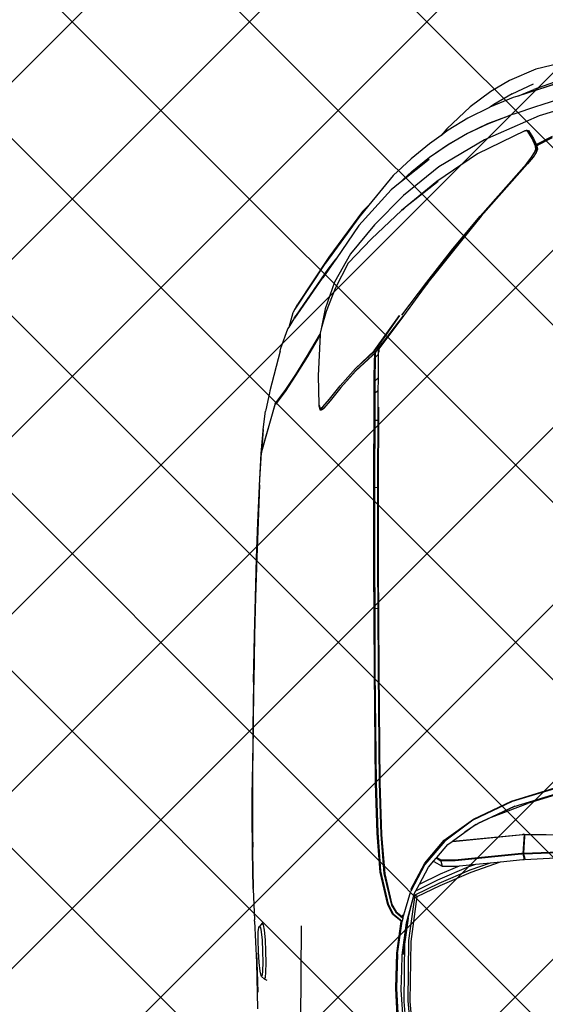
# Model space of a CAD drawing. Units: inches. Extents: x 2167 to 2589, y 1680 to 2489.
# Tile 25 of 38: x 2335 to 2356, y 1796 to 1835. Entities that reach past the tile are written whole.
import ezdxf

# ---------------------------------------------------------------- set-up
doc = ezdxf.new("R2010")
doc.units = ezdxf.units.IN
doc.header["$MEASUREMENT"] = 0
doc.layers.get('0').update_dxf_attribs({"color": 250})
doc.layers.add('C-PRKG-VEHS', color=8, linetype='Continuous', lineweight=13)
doc.layers.add('L-PVMT-PATT', color=252, linetype='Continuous', lineweight=13)
doc.layers.add('Edges', color=250, linetype='Continuous')

# ---------------------------------------------------------------- blocks, each defined once
blk = doc.blocks.new('Nissan Qashqai pl')
at = {"layer": 'Edges'}
for p, q in [((8.4086, 11.6764), (8.4045, 11.4011)), ((8.4305, 11.3996), (8.419, 11.6758)), ((8.4204, 11.6758), (8.4319, 11.3996)), ((8.4394, 11.4014), (8.4238, 11.6766)), ((7.3676, 11.5172), (7.3963, 11.4215)), ((8.3392, 11.4758), (8.3608, 11.4048)), ((7.3193, 11.4645), (7.3309, 11.4166)), ((8.3573, 11.3824), (8.3296, 11.4739)), ((8.3311, 11.4733), (8.3582, 11.3836)), ((8.3648, 11.3863), (8.3377, 11.4753)), ((7.344, 11.4572), (7.3596, 11.4139)), ((7.3467, 11.4596), (7.3686, 11.3913)), ((7.3489, 11.4517), (7.3686, 11.3913)), ((7.375, 11.4442), (7.3799, 11.4278)), ((7.4255, 11.4398), (7.4367, 11.4174)), ((7.4379, 11.4179), (7.4267, 11.4401)), ((8.4041, 11.4013), (8.4048, 11.4423)), ((7.3799, 11.4278), (7.3845, 11.4136)), ((7.3963, 11.4215), (7.4302, 11.3449)), ((7.3309, 11.4166), (7.347, 11.3798)), ((7.3655, 11.3837), (7.3514, 11.4133)), ((7.3686, 11.3913), (7.3596, 11.4139)), ((7.3845, 11.4136), (7.3925, 11.3899)), ((7.4282, 11.4113), (7.4169, 11.4044)), ((7.417, 11.4065), (7.4283, 11.4135)), ((7.4296, 11.4129), (7.4183, 11.406)), ((7.4387, 11.4162), (7.4282, 11.4113)), ((7.4283, 11.4135), (7.4359, 11.417)), ((7.4296, 11.4129), (7.4383, 11.417)), ((7.4359, 11.417), (7.4367, 11.4174)), ((7.4383, 11.417), (7.4367, 11.4174)), ((7.4375, 11.42), (7.4384, 11.4182)), ((7.4379, 11.4179), (7.4384, 11.4182)), ((7.4389, 11.4173), (7.4379, 11.4179)), ((7.4383, 11.417), (7.4379, 11.4179)), ((7.4389, 11.4173), (7.4383, 11.417)), ((7.4384, 11.4182), (7.4387, 11.4183)), ((7.4387, 11.4183), (7.443, 11.4188)), ((7.4431, 11.4166), (7.4387, 11.4162)), ((7.4389, 11.4173), (7.44, 11.4178)), ((7.4442, 11.4183), (7.44, 11.4178)), ((7.443, 11.4188), (7.4477, 11.4172)), ((7.4479, 11.4149), (7.4431, 11.4166)), ((7.4477, 11.4172), (7.4442, 11.4183)), ((7.4477, 11.4172), (7.4541, 11.4128)), ((7.4541, 11.4108), (7.4479, 11.4149)), ((7.4541, 11.4128), (7.4638, 11.4051)), ((7.4635, 11.4034), (7.4541, 11.4108)), ((7.4167, 11.4049), (7.417, 11.4065)), ((7.4172, 11.4047), (7.4167, 11.4049)), ((7.4169, 11.4036), (7.4167, 11.4049)), ((7.4172, 11.4047), (7.4169, 11.4044)), ((7.4169, 11.4044), (7.4169, 11.4036)), ((7.4172, 11.4018), (7.4169, 11.4036)), ((7.4169, 11.4036), (7.4169, 11.403)), ((7.4169, 11.403), (7.4172, 11.4011)), ((7.4183, 11.406), (7.4172, 11.4047)), ((7.4174, 11.4013), (7.4172, 11.4018)), ((7.4172, 11.4011), (7.4498, 11.3349)), ((7.4174, 11.4013), (7.4175, 11.4012)), ((7.5369, 11.3385), (7.4635, 11.4034)), ((7.4638, 11.4051), (7.5371, 11.34)), ((8.3799, 11.3545), (8.3608, 11.4048)), ((8.407, 11.401), (8.4037, 11.4002)), ((8.4037, 11.4002), (8.4314, 11.3985)), ((8.4037, 11.3992), (8.4037, 11.4002)), ((8.4037, 11.3992), (8.4046, 11.3981)), ((8.4042, 11.3983), (8.4037, 11.3992)), ((8.4041, 11.4013), (8.4045, 11.4011)), ((8.4134, 11.3049), (8.4042, 11.3983)), ((8.4045, 11.4011), (8.407, 11.401)), ((8.4046, 11.3981), (8.4138, 11.3048)), ((8.407, 11.401), (8.4305, 11.3996)), ((8.4305, 11.3996), (8.4319, 11.3996)), ((8.4306, 11.3966), (8.4314, 11.3975)), ((8.4398, 11.3032), (8.4306, 11.3966)), ((8.4314, 11.3985), (8.4394, 11.4004)), ((8.4314, 11.3985), (8.4314, 11.3975)), ((8.4314, 11.3975), (8.4319, 11.3967)), ((8.4319, 11.3996), (8.436, 11.4006)), ((8.4319, 11.3967), (8.4412, 11.3033)), ((8.436, 11.4006), (8.4394, 11.4014)), ((8.4394, 11.4004), (8.436, 11.4006)), ((8.4394, 11.3984), (8.4394, 11.4004)), ((8.4425, 11.3672), (8.4394, 11.3984)), ((7.347, 11.3798), (7.3624, 11.3535)), ((7.3655, 11.3837), (7.3805, 11.3576)), ((7.3686, 11.3913), (7.3707, 11.3849)), ((7.3707, 11.3849), (7.3843, 11.3522)), ((7.3925, 11.3899), (7.3938, 11.3859)), ((7.3938, 11.3859), (7.3951, 11.3822)), ((7.3951, 11.3822), (7.3965, 11.3787)), ((8.3826, 11.3291), (8.3573, 11.3824)), ((8.3582, 11.3836), (8.3844, 11.3284)), ((8.3646, 11.387), (8.3799, 11.3545)), ((8.3888, 11.3355), (8.3648, 11.3863)), ((7.3962, 11.3781), (7.3965, 11.3787)), ((7.4071, 11.3493), (7.3962, 11.3781)), ((7.3965, 11.3787), (7.3969, 11.3777)), ((7.3969, 11.3777), (7.4078, 11.349)), ((8.4571, 11.3258), (8.4425, 11.3672)), ((8.4439, 11.3531), (8.4425, 11.3672)), ((7.3624, 11.3535), (7.3837, 11.3245)), ((7.3805, 11.3576), (7.3843, 11.3522)), ((7.3843, 11.3522), (7.3845, 11.3517)), ((7.3845, 11.3517), (7.3997, 11.3215)), ((8.3799, 11.3545), (8.3888, 11.3355)), ((8.454, 11.3245), (8.4439, 11.3531)), ((8.4459, 11.3326), (8.4439, 11.3531)), ((7.4205, 11.3212), (7.4071, 11.3493)), ((7.4078, 11.349), (7.4211, 11.321)), ((7.4302, 11.3449), (7.4679, 11.2807)), ((7.5827, 11.3001), (7.5369, 11.3385)), ((7.5371, 11.34), (7.5568, 11.324)), ((7.3837, 11.3245), (7.4147, 11.2918)), ((7.4498, 11.3349), (7.4884, 11.2778)), ((7.584, 11.3013), (7.5568, 11.324)), ((7.5568, 11.324), (7.5829, 11.303)), ((8.4122, 11.2883), (8.3826, 11.3291)), ((8.3844, 11.3284), (8.4134, 11.2888)), ((8.3901, 11.3328), (8.3888, 11.3355)), ((8.3901, 11.3328), (8.4011, 11.3173)), ((8.3904, 11.3321), (8.3901, 11.3328)), ((8.4011, 11.3173), (8.3904, 11.3321)), ((8.4493, 11.3229), (8.4459, 11.3326)), ((8.4482, 11.3095), (8.4459, 11.3326)), ((8.4725, 11.2812), (8.454, 11.3245)), ((8.4756, 11.2826), (8.4571, 11.3258)), ((7.3997, 11.3215), (7.4166, 11.2939)), ((7.4363, 11.294), (7.4205, 11.3212)), ((7.4211, 11.321), (7.4369, 11.2938)), ((8.4135, 11.3), (8.4011, 11.3173)), ((8.468, 11.2793), (8.4493, 11.3229)), ((7.6296, 11.2639), (7.5827, 11.3001)), ((7.5829, 11.303), (7.618, 11.275)), ((7.618, 11.275), (7.584, 11.3013)), ((8.4135, 11.3), (8.4134, 11.3049)), ((8.4139, 11.2994), (8.4135, 11.3)), ((8.4138, 11.3048), (8.4139, 11.2994)), ((8.4183, 11.2934), (8.4139, 11.2994)), ((8.44, 11.2834), (8.4398, 11.3032)), ((8.4412, 11.3033), (8.4415, 11.2835)), ((8.4594, 11.2831), (8.4482, 11.3095)), ((8.4487, 11.305), (8.4482, 11.3095)), ((8.4489, 11.2852), (8.4487, 11.305)), ((7.4147, 11.2918), (7.4239, 11.2837)), ((7.4166, 11.2939), (7.4239, 11.2837)), ((7.4239, 11.2837), (7.4354, 11.2675)), ((7.4542, 11.2677), (7.4363, 11.294)), ((7.4369, 11.2938), (7.4549, 11.2675)), ((8.4444, 11.2608), (8.4122, 11.2883)), ((8.4134, 11.2888), (8.4462, 11.2609)), ((8.4365, 11.2776), (8.4183, 11.2934)), ((8.4365, 11.2776), (8.44, 11.2834)), ((8.4415, 11.2835), (8.4375, 11.2767)), ((8.4415, 11.2835), (8.4489, 11.2852)), ((8.4422, 11.2737), (8.4489, 11.2852)), ((8.4737, 11.2534), (8.4594, 11.2831)), ((8.4914, 11.25), (8.4756, 11.2826)), ((7.4679, 11.2807), (7.5081, 11.2311)), ((7.4882, 11.2797), (7.5243, 11.2341)), ((7.4884, 11.2778), (7.5289, 11.2283)), ((7.618, 11.275), (7.6301, 11.2654)), ((8.4375, 11.2767), (8.4365, 11.2776)), ((8.4412, 11.2735), (8.4375, 11.2767)), ((8.4422, 11.2737), (8.4412, 11.2735)), ((8.4499, 11.2659), (8.4412, 11.2735)), ((8.4831, 11.2484), (8.468, 11.2793)), ((8.4889, 11.2473), (8.4725, 11.2812)), ((7.4354, 11.2675), (7.4565, 11.2419)), ((7.4744, 11.2427), (7.4542, 11.2677)), ((7.4549, 11.2675), (7.475, 11.2426)), ((7.4574, 11.267), (7.4885, 11.2283)), ((7.676, 11.2289), (7.6296, 11.2639)), ((7.6301, 11.2654), (7.6306, 11.2651)), ((7.6306, 11.2651), (7.6306, 11.265)), ((7.6306, 11.265), (7.6373, 11.2601)), ((7.6373, 11.2601), (7.6769, 11.2312)), ((8.4814, 11.2413), (8.4444, 11.2608)), ((8.4462, 11.2609), (8.4838, 11.2415)), ((8.4737, 11.2534), (8.4499, 11.2659)), ((7.4565, 11.2419), (7.4801, 11.2168)), ((7.4918, 11.2242), (7.4744, 11.2427)), ((7.475, 11.2426), (7.477, 11.2404)), ((7.477, 11.2404), (7.4765, 11.2411)), ((8.4831, 11.2484), (8.4737, 11.2534)), ((8.4867, 11.2465), (8.4831, 11.2484)), ((8.5216, 11.2303), (8.4838, 11.2415)), ((8.528, 11.2354), (8.4867, 11.2465)), ((8.5214, 11.2374), (8.4867, 11.2465)), ((8.4889, 11.2473), (8.4914, 11.25)), ((8.5531, 11.2387), (8.4889, 11.2473)), ((8.5544, 11.2416), (8.4914, 11.25)), ((8.6386, 11.2404), (8.5544, 11.2416)), ((8.7481, 11.2473), (8.6375, 11.2376)), ((8.7491, 11.2501), (8.6386, 11.2404)), ((7.477, 11.2405), (7.4775, 11.2399)), ((7.4784, 11.2388), (7.477, 11.2404)), ((7.477, 11.2404), (7.4775, 11.2399)), ((7.4775, 11.2399), (7.4787, 11.2385)), ((7.4775, 11.2399), (7.4787, 11.2387)), ((7.4787, 11.2387), (7.4782, 11.2392)), ((7.4795, 11.2377), (7.4787, 11.2387)), ((7.4787, 11.2387), (7.4885, 11.2283)), ((7.4885, 11.2283), (7.4918, 11.2242)), ((7.5081, 11.2311), (7.5492, 11.1902)), ((7.5243, 11.2341), (7.5286, 11.2296)), ((7.5289, 11.2283), (7.5687, 11.1862)), ((7.6769, 11.2312), (7.7194, 11.1992)), ((7.7232, 11.1955), (7.6771, 11.2307)), ((8.5125, 11.221), (8.5177, 11.2272)), ((8.5132, 11.2202), (8.5216, 11.2303)), ((8.5155, 11.2168), (8.5258, 11.2291)), ((8.5197, 11.2297), (8.5166, 11.2307)), ((8.5177, 11.2272), (8.5197, 11.2297)), ((8.5216, 11.2303), (8.5197, 11.2297)), ((8.5214, 11.2374), (8.555, 11.233)), ((8.5301, 11.2352), (8.5214, 11.2374)), ((8.5216, 11.2303), (8.5258, 11.2291)), ((8.5259, 11.2279), (8.5237, 11.2252)), ((8.5258, 11.2291), (8.5259, 11.2279)), ((8.5715, 11.2227), (8.5258, 11.2291)), ((8.5294, 11.2274), (8.5259, 11.2279)), ((8.5736, 11.2291), (8.528, 11.2354)), ((8.5706, 11.2216), (8.5294, 11.2274)), ((8.6375, 11.2376), (8.5531, 11.2387)), ((8.6387, 11.2319), (8.555, 11.233)), ((8.555, 11.233), (8.5726, 11.2307)), ((8.5941, 11.2286), (8.5736, 11.2291)), ((8.5941, 11.2289), (8.5941, 11.2286)), ((8.622, 11.228), (8.5941, 11.2286)), ((8.6699, 11.231), (8.622, 11.228)), ((8.6721, 11.2348), (8.6387, 11.2319)), ((7.4801, 11.2168), (7.5217, 11.1823)), ((7.4918, 11.2242), (7.5001, 11.2139)), ((7.5001, 11.2139), (7.5501, 11.1684)), ((7.7261, 11.1898), (7.6762, 11.2256)), ((7.6762, 11.2256), (7.7233, 11.1928)), ((8.4588, 11.2036), (8.5032, 11.2141)), ((8.4595, 11.2047), (8.5025, 11.2148)), ((8.5155, 11.2168), (8.5018, 11.2098)), ((8.5025, 11.2148), (8.5125, 11.221)), ((8.5163, 11.2162), (8.5029, 11.2092)), ((8.5032, 11.2141), (8.5132, 11.2202)), ((8.5237, 11.2252), (8.5163, 11.2162)), ((8.6197, 11.2201), (8.5706, 11.2216)), ((8.5715, 11.2227), (8.6203, 11.2213)), ((8.6683, 11.2226), (8.6197, 11.2201)), ((8.6203, 11.2213), (8.6721, 11.2241)), ((8.3318, 11.198), (8.4049, 11.2004)), ((8.332, 11.1971), (8.4042, 11.1995)), ((8.4042, 11.1995), (8.4588, 11.2036)), ((8.4049, 11.2004), (8.4595, 11.2047)), ((8.5018, 11.2098), (8.4559, 11.1991)), ((8.5029, 11.2092), (8.4571, 11.1983)), ((7.5492, 11.1902), (7.59, 11.1565)), ((7.5687, 11.1862), (7.6032, 11.1533)), ((7.7194, 11.1992), (7.7232, 11.1966)), ((7.7232, 11.1966), (7.7279, 11.1965)), ((7.7281, 11.1918), (7.7232, 11.1955)), ((7.7232, 11.1955), (7.7245, 11.1955)), ((7.7267, 11.1902), (7.7233, 11.1928)), ((7.7247, 11.1954), (7.7245, 11.1955)), ((7.7245, 11.1955), (7.7294, 11.1955)), ((7.7261, 11.1898), (7.7507, 11.1638)), ((7.7286, 11.1881), (7.7267, 11.1902)), ((7.7281, 11.1918), (7.7299, 11.1904)), ((7.7349, 11.1917), (7.7281, 11.1918)), ((7.753, 11.1648), (7.7281, 11.1918)), ((7.7507, 11.1638), (7.7286, 11.1881)), ((7.7294, 11.1955), (7.731, 11.1955)), ((7.7299, 11.1904), (7.7324, 11.1876)), ((7.7299, 11.1904), (7.7364, 11.1904)), ((7.731, 11.1955), (7.7349, 11.1917)), ((7.731, 11.1955), (7.764, 11.1953)), ((7.7324, 11.1876), (7.7539, 11.1642)), ((7.768, 11.1915), (7.7349, 11.1917)), ((7.7363, 11.1904), (7.7364, 11.1904)), ((7.7694, 11.1901), (7.7364, 11.1904)), ((7.764, 11.1953), (7.7636, 11.1957)), ((7.768, 11.1915), (7.764, 11.1953)), ((7.764, 11.1953), (7.7662, 11.1953)), ((7.7659, 11.1957), (7.7662, 11.1953)), ((7.7662, 11.1953), (7.7668, 11.1946)), ((7.7662, 11.1953), (7.7811, 11.1952)), ((7.7692, 11.1915), (7.768, 11.1915)), ((7.7694, 11.1901), (7.7687, 11.1908)), ((7.7844, 11.1913), (7.7692, 11.1915)), ((7.7707, 11.1901), (7.7694, 11.1901)), ((7.7851, 11.19), (7.7707, 11.1901)), ((7.7811, 11.1952), (7.7809, 11.1958)), ((7.7814, 11.1946), (7.7811, 11.1952)), ((7.7811, 11.1952), (7.7822, 11.1952)), ((7.7822, 11.1952), (7.7819, 11.1958)), ((7.7822, 11.1952), (7.8057, 11.195)), ((7.7844, 11.1913), (7.7822, 11.1952)), ((7.8078, 11.1911), (7.7844, 11.1913)), ((7.7846, 11.1909), (7.7851, 11.19)), ((7.8083, 11.1898), (7.7851, 11.19)), ((7.8048, 11.1959), (7.8233, 11.1958)), ((7.8057, 11.195), (7.8233, 11.195)), ((7.8233, 11.1911), (7.8078, 11.1911)), ((7.904, 11.1894), (7.8083, 11.1898)), ((7.8233, 11.195), (7.8233, 11.1958)), ((7.8233, 11.1958), (7.9014, 11.1955)), ((7.8233, 11.195), (7.902, 11.1947)), ((7.8233, 11.1911), (7.8233, 11.195)), ((7.8233, 11.1899), (7.8233, 11.1911)), ((7.9036, 11.1907), (7.8233, 11.1911)), ((7.9014, 11.1955), (7.9185, 11.1955)), ((7.902, 11.1947), (7.9183, 11.1947)), ((7.9176, 11.1908), (7.9036, 11.1907)), ((8.0276, 11.1896), (7.904, 11.1894)), ((7.9183, 11.1947), (7.9176, 11.1908)), ((8.0275, 11.1909), (7.9176, 11.1908)), ((7.9185, 11.1955), (7.9183, 11.1947)), ((7.9183, 11.1947), (8.0275, 11.1948)), ((7.9185, 11.1955), (8.0273, 11.1957)), ((8.0273, 11.1957), (8.1753, 11.1963)), ((8.0275, 11.1948), (8.0876, 11.1951)), ((8.0873, 11.1911), (8.0275, 11.1909)), ((8.1753, 11.1903), (8.0276, 11.1896)), ((8.0876, 11.1951), (8.0873, 11.1911)), ((8.1755, 11.1915), (8.0873, 11.1911)), ((8.0876, 11.1951), (8.1754, 11.1954)), ((8.1753, 11.1963), (8.3318, 11.198)), ((8.3324, 11.192), (8.1753, 11.1903)), ((8.1754, 11.1954), (8.332, 11.1971)), ((8.3324, 11.1931), (8.1755, 11.1915)), ((8.4014, 11.1953), (8.3324, 11.1931)), ((8.4022, 11.1943), (8.3324, 11.192)), ((8.4559, 11.1991), (8.4014, 11.1953)), ((8.4571, 11.1983), (8.4022, 11.1943)), ((7.5304, 11.1737), (7.5217, 11.1823)), ((7.5217, 11.1823), (7.5387, 11.1682)), ((7.5304, 11.1737), (7.5946, 11.1262)), ((7.5387, 11.1682), (7.6031, 11.1217)), ((7.5501, 11.1684), (7.5969, 11.1365)), ((7.7748, 11.1423), (7.7507, 11.1638)), ((7.753, 11.1648), (7.7772, 11.1431)), ((7.7539, 11.1642), (7.7772, 11.1431)), ((7.59, 11.1565), (7.6295, 11.1344)), ((7.6032, 11.1533), (7.6386, 11.1353)), ((7.6113, 11.1256), (7.5969, 11.1365)), ((7.5969, 11.1365), (7.6021, 11.1329)), ((7.6021, 11.1329), (7.6118, 11.1255)), ((7.6021, 11.1329), (7.6237, 11.1181)), ((7.6295, 11.1344), (7.667, 11.1212)), ((7.6386, 11.1353), (7.6708, 11.1225)), ((7.7938, 11.1271), (7.7748, 11.1423)), ((7.7772, 11.1431), (7.7959, 11.1281)), ((7.5946, 11.1262), (7.6608, 11.0825)), ((7.6676, 11.0791), (7.6024, 11.1221)), ((7.6759, 11.0809), (7.6113, 11.1256)), ((7.6118, 11.1255), (7.6799, 11.0783)), ((7.667, 11.1212), (7.6949, 11.1158)), ((7.6708, 11.1225), (7.6949, 11.1158)), ((7.8045, 11.1179), (7.7938, 11.1271)), ((7.7959, 11.1281), (7.8062, 11.1192)), ((7.8072, 11.1141), (7.8045, 11.1179)), ((7.8087, 11.1159), (7.8062, 11.1192)), ((7.8062, 11.1192), (7.8066, 11.1188)), ((7.8066, 11.1188), (7.8096, 11.1148)), ((7.6949, 11.1158), (7.701, 11.1141)), ((7.701, 11.1141), (7.7024, 11.1141)), ((7.7038, 11.1132), (7.7024, 11.1141)), ((7.7024, 11.1141), (7.7034, 11.114)), ((7.7034, 11.114), (7.7056, 11.1128)), ((7.7034, 11.114), (7.7608, 11.1112)), ((7.7325, 11.0966), (7.7038, 11.1132)), ((7.7056, 11.1128), (7.7341, 11.0963)), ((7.7608, 11.1112), (7.8014, 11.1124)), ((7.8014, 11.1124), (7.8022, 11.1126)), ((7.8022, 11.1126), (7.8072, 11.1141)), ((7.8037, 11.1126), (7.8022, 11.1126)), ((7.8096, 11.1148), (7.8037, 11.1126)), ((7.8072, 11.1141), (7.8087, 11.1159)), ((7.7591, 11.08), (7.7325, 11.0966)), ((7.7341, 11.0963), (7.7606, 11.0798)), ((7.6712, 11.0767), (7.6608, 11.0825)), ((7.6721, 11.0762), (7.6712, 11.0767)), ((7.6926, 11.0705), (7.6721, 11.0762)), ((7.6793, 11.0784), (7.6759, 11.0809)), ((7.6802, 11.0782), (7.6793, 11.0784)), ((7.6802, 11.0782), (7.6799, 11.0783)), ((7.6809, 11.0777), (7.6802, 11.0782)), ((7.6926, 11.0705), (7.6809, 11.0777)), ((7.7814, 11.065), (7.7591, 11.08)), ((7.7606, 11.0798), (7.7828, 11.0649)), ((8.5326, 11.0874), (8.6675, 11.0866)), ((7.6953, 11.0688), (7.6926, 11.0705)), ((7.7223, 11.059), (7.6953, 11.0688)), ((7.797, 11.0534), (7.7814, 11.065)), ((7.7828, 11.0649), (7.7984, 11.0533)), ((7.7262, 11.0581), (7.7223, 11.059)), ((7.7262, 11.0581), (7.7819, 11.0438)), ((7.797, 11.0534), (7.797, 11.0534)), ((7.7998, 11.0513), (7.797, 11.0534)), ((7.7984, 11.0533), (7.8007, 11.0516)), ((7.7998, 11.0513), (7.8676, 11.0318)), ((7.8007, 11.0516), (7.8002, 11.0517)), ((7.8007, 11.0516), (7.8012, 11.0513)), ((7.8681, 11.032), (7.8012, 11.0513)), ((7.7819, 11.0438), (7.7848, 11.043)), ((7.7848, 11.043), (7.8087, 11.038)), ((7.8087, 11.038), (7.8106, 11.0377)), ((7.8107, 11.0377), (7.8106, 11.0377)), ((7.8363, 11.0344), (7.8107, 11.0377)), ((7.8381, 11.0342), (7.8363, 11.0344)), ((7.8363, 11.0344), (7.8676, 11.0318)), ((7.87, 11.0315), (7.8381, 11.0342)), ((8.531, 11.0346), (8.5287, 11.0329)), ((8.5385, 11.0363), (8.531, 11.0346)), ((8.5518, 11.0375), (8.5385, 11.0363)), ((8.568, 11.0382), (8.5518, 11.0375)), ((8.5842, 11.0384), (8.568, 11.0382)), ((8.5681, 11.0335), (8.5836, 11.0337)), ((8.5836, 11.0337), (8.5957, 11.0334)), ((8.5974, 11.0381), (8.5842, 11.0384)), ((8.6049, 11.0373), (8.5974, 11.0381)), ((8.6073, 11.0362), (8.6032, 11.0321)), ((8.6073, 11.0362), (8.6049, 11.0373)), ((8.609, 11.0397), (8.6073, 11.0362)), ((7.8681, 11.032), (7.8676, 11.0318)), ((7.8681, 11.032), (7.869, 11.0317)), ((7.9137, 11.0292), (7.869, 11.0317)), ((7.9151, 11.029), (7.87, 11.0315)), ((7.9137, 11.0292), (7.9658, 11.027)), ((7.9668, 11.0268), (7.9151, 11.029)), ((7.9658, 11.027), (8.016, 11.0253)), ((8.0168, 11.0251), (7.9668, 11.0268)), ((8.016, 11.0253), (8.0713, 11.0237)), ((8.0718, 11.0235), (8.0168, 11.0251)), ((8.0713, 11.0237), (8.1249, 11.0223)), ((8.1251, 11.0222), (8.0718, 11.0235)), ((8.1249, 11.0223), (8.1901, 11.021)), ((8.1902, 11.0208), (8.1251, 11.0222)), ((8.1901, 11.021), (8.1938, 11.021)), ((8.1902, 11.021), (8.1938, 11.021)), ((8.1904, 11.0209), (8.1902, 11.0208)), ((8.1904, 11.0209), (8.2543, 11.0198)), ((8.1938, 11.021), (8.1954, 11.0209)), ((8.1954, 11.0209), (8.2544, 11.02)), ((8.2544, 11.02), (8.3166, 11.0193)), ((8.4799, 11.0202), (8.4282, 11.0193)), ((8.4292, 11.0193), (8.4799, 11.0202)), ((8.4811, 11.0203), (8.4799, 11.0202)), ((8.4811, 11.0203), (8.5241, 11.022)), ((8.5259, 11.0221), (8.5241, 11.022)), ((8.5259, 11.0221), (8.5838, 11.0251)), ((8.5283, 11.0336), (8.5287, 11.0329)), ((8.5287, 11.0329), (8.5331, 11.0292)), ((8.5331, 11.0292), (8.5346, 11.0303)), ((8.5347, 11.0282), (8.5331, 11.0292)), ((8.5346, 11.0303), (8.5406, 11.0316)), ((8.5407, 11.0274), (8.5347, 11.0282)), ((8.5406, 11.0316), (8.5526, 11.0328)), ((8.5527, 11.0273), (8.5407, 11.0274)), ((8.5526, 11.0328), (8.5681, 11.0335)), ((8.5682, 11.0278), (8.5527, 11.0273)), ((8.5837, 11.0288), (8.5682, 11.0278)), ((8.5707, 11.0248), (8.5965, 11.0258)), ((8.5958, 11.0301), (8.5837, 11.0288)), ((8.5838, 11.0251), (8.6489, 11.0263)), ((8.5838, 11.0251), (8.5965, 11.0258)), ((8.5957, 11.0334), (8.6017, 11.0328)), ((8.6018, 11.0312), (8.5958, 11.0301)), ((8.5965, 11.0258), (8.6252, 11.0268)), ((8.6017, 11.0328), (8.6032, 11.0321)), ((8.6032, 11.0321), (8.6018, 11.0312)), ((8.2544, 11.0198), (8.2543, 11.0199)), ((8.2543, 11.0198), (8.2544, 11.0198)), ((8.2544, 11.0198), (8.2556, 11.0198)), ((8.2556, 11.0198), (8.256, 11.0198)), ((8.256, 11.0198), (8.2561, 11.0198)), ((8.2561, 11.0198), (8.2693, 11.0197)), ((8.2693, 11.0197), (8.2694, 11.0197)), ((8.2694, 11.0197), (8.3098, 11.0192)), ((8.3098, 11.0192), (8.3163, 11.0192)), ((8.3663, 11.019), (8.3163, 11.0192)), ((8.3597, 11.019), (8.3163, 11.0192)), ((8.3166, 11.0193), (8.3764, 11.0191)), ((8.3602, 11.019), (8.3597, 11.019)), ((8.3608, 11.019), (8.3602, 11.019)), ((8.3663, 11.019), (8.3608, 11.019)), ((8.3663, 11.019), (8.3764, 11.0191)), ((8.3757, 11.019), (8.3663, 11.019)), ((8.4282, 11.0193), (8.3757, 11.019)), ((8.3764, 11.0191), (8.4069, 11.0192)), ((8.4069, 11.0192), (8.4219, 11.0196)), ((8.4069, 11.0192), (8.4292, 11.0193))]:
    blk.add_line(p, q, dxfattribs=at)
blk = doc.blocks.new('car')
blk.add_blockref('Nissan Qashqai pl', (-9.7433, -11.9151))
blk = doc.blocks.new('carr')
blk.add_blockref('car', (0.5124, -0.007))

msp = doc.modelspace()

# ---------------------------------------------------------------- hatches: boundary and pattern name
at = {"layer": 'L-PVMT-PATT'}
h = msp.add_hatch(dxfattribs=at)
h.set_pattern_fill('ANSI37', color=256, scale=40)
h.paths.add_polyline_path([(2417.548, 1783.695), (2417.548, 1846.042), (2239.361, 1846.042), (2239.361, 1687.695), (2369.843, 1687.695), (2369.843, 1696.695), (2375.607, 1696.695), (2416.107, 1696.695), (2417.548, 1696.695)])

# ---------------------------------------------------------------- block references
at = {"layer": 'C-PRKG-VEHS', "xscale": 28.42784210623918, "yscale": 28.42784210623918, "zscale": 28.42784210623918, "rotation": 270}
msp.add_blockref('carr', (2369.852, 1779.037), dxfattribs=at)

doc.saveas('drawing.dxf')
